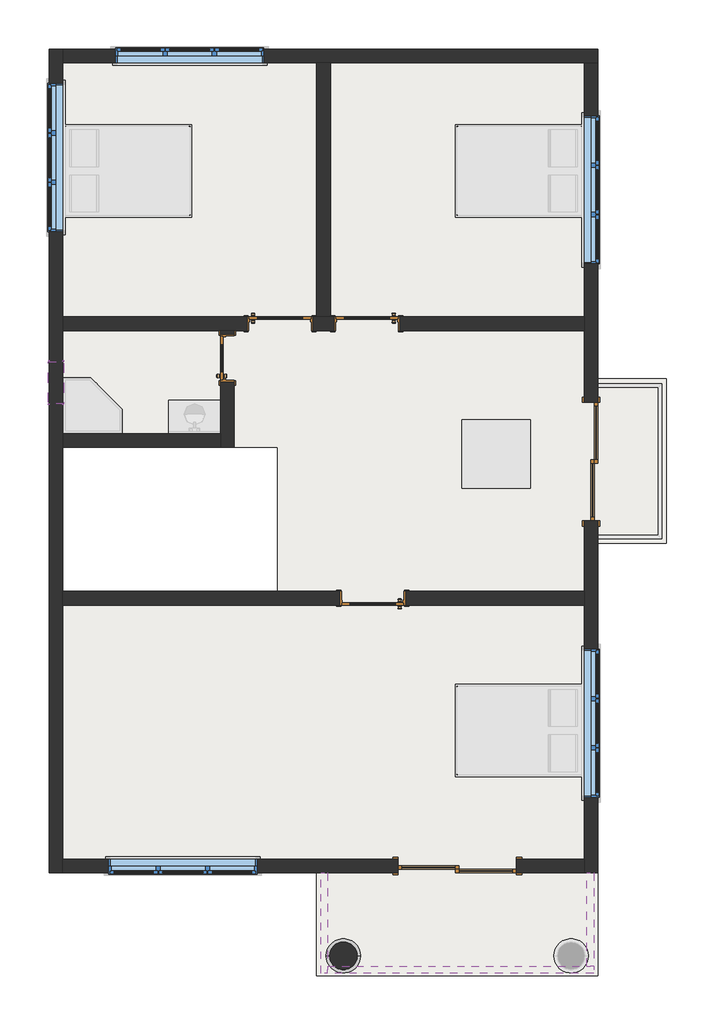
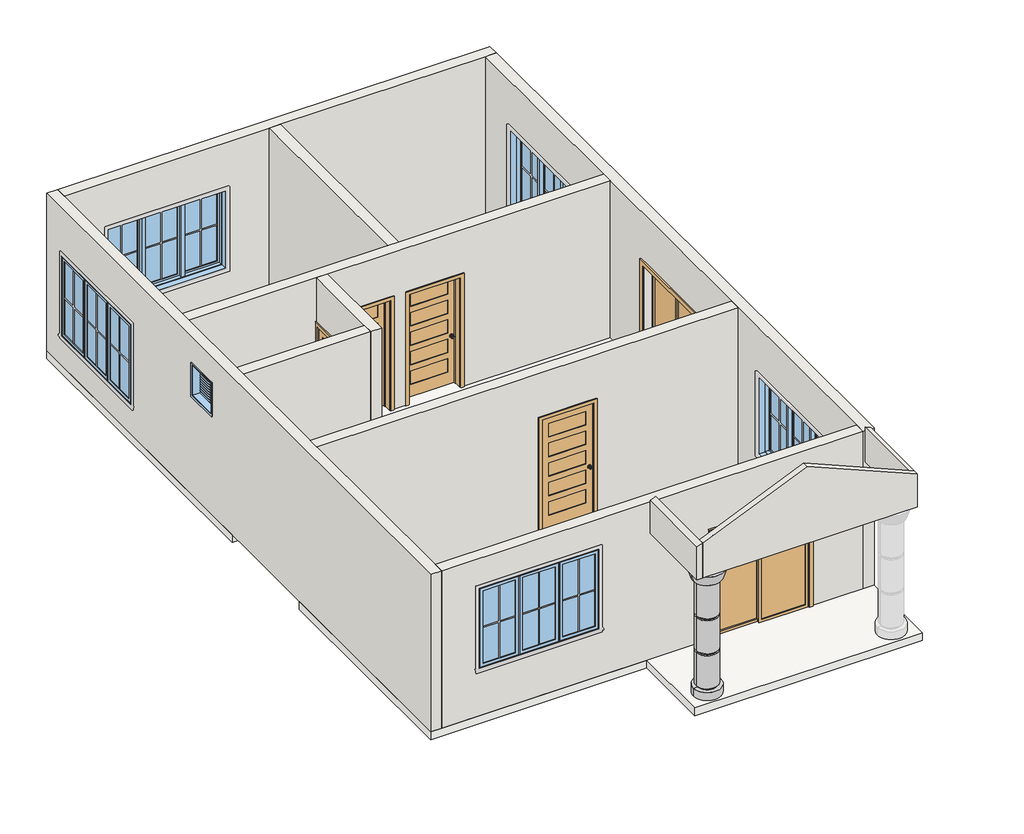
# One storey, part 1 of 2: 12 walls, 6 doors, 6 windows, 1 column, 1 slab.
"""IFC4 building model written with IfcOpenShell, lengths in millimetres."""

from ifc_helpers import new_model, si_unit, frame, origin, place, context, project, spatial, polyline, circle_curve, outline, extrude, faceted_brep, transform, mapped, element, save
from ifc_brep_helpers import plane_surface, cylinder_surface, revolved_surface, advanced_brep
from components import door_e30895c2, door_3f7a11fd, door_bc447172, door_interior_single_5_panel_vert_wood_650_x_2100_a7f2c8da, window_45599283, window_35a91c22

model = new_model("IFC4")

# Units and contexts
model_context = context("Model", 3, world=origin())
ifc_project = project(units=[si_unit("LENGTHUNIT", "METRE", prefix="MILLI")], contexts=[model_context])

# Site, building, storey
site = spatial("IfcSite", under=ifc_project)
building = spatial("IfcBuilding", under=site)
storey = spatial("IfcBuildingStorey", under=building, Elevation=3400.0)

# Column
placement = place(None, origin())
element("IfcColumn", 1, ObjectType="Metal Clad Column : 400MM COLUMN", at=placement, inside=storey, context=model_context, shape_type="AdvancedBrep", body=[
    advanced_brep(
    [(-1050.7658003, -5475.1432863, 3400.0), (-1301.5658003, -5475.1432863, 3400.0), (-799.9658003, -5475.1432863, 3400.0), (-1301.5658003, -5475.1432863, 3552.4), (-799.9658003, -5475.1432863, 3552.4), (-876.1658003, -5475.1432863, 4259.2666667), (-1225.3658003, -5475.1432863, 4259.2666667), (-1250.7658003, -5475.1432863, 4259.2666667), (-850.7658003, -5475.1432863, 4259.2666667), (-1250.7658003, -5475.1432863, 4889.9333333), (-850.7658003, -5475.1432863, 4889.9333333), (-876.1658003, -5475.1432863, 4221.1666667), (-1225.3658003, -5475.1432863, 4221.1666667), (-850.7658003, -5475.1432863, 4221.1666667), (-1250.7658003, -5475.1432863, 4221.1666667), (-850.7658003, -5475.1432863, 3590.5), (-1250.7658003, -5475.1432863, 3590.5), (-876.1658003, -5475.1432863, 3590.5), (-1225.3658003, -5475.1432863, 3590.5), (-876.1658003, -5475.1432863, 3552.4), (-1225.3658003, -5475.1432863, 3552.4), (-799.9658003, -5475.1432863, 5596.8), (-1301.5658003, -5475.1432863, 5596.8), (-1365.0658003, -5475.1432863, 5800.0), (-736.4658003, -5475.1432863, 5800.0), (-1050.7658003, -5475.1432863, 5800.0), (-876.1658003, -5475.1432863, 5596.8), (-1225.3658003, -5475.1432863, 5596.8), (-876.1658003, -5475.1432863, 5558.7), (-1225.3658003, -5475.1432863, 5558.7), (-850.7658003, -5475.1432863, 5558.7), (-1250.7658003, -5475.1432863, 5558.7), (-850.7658003, -5475.1432863, 4928.0333333), (-1250.7658003, -5475.1432863, 4928.0333333), (-876.1658003, -5475.1432863, 4928.0333333), (-1225.3658003, -5475.1432863, 4928.0333333), (-876.1658003, -5475.1432863, 4889.9333333), (-1225.3658003, -5475.1432863, 4889.9333333)],
    [
        (0, 1),
        (1, 2, circle_curve(frame((-1050.7658003, -5475.1432863, 3400.0), z_axis=(0.0, 0.0, -1.0), x_axis=(-1.0, 0.0, 0.0)), 250.8)),
        (2, 0),
        (2, 1, circle_curve(frame((-1050.7658003, -5475.1432863, 3400.0), z_axis=(0.0, 0.0, -1.0), x_axis=(-1.0, 0.0, 0.0)), 250.8)),
        (1, 3),
        (3, 4, circle_curve(frame((-1050.7658003, -5475.1432863, 3552.4), z_axis=(0.0, 0.0, -1.0), x_axis=(-1.0, 0.0, 0.0)), 250.8)),
        (4, 2),
        (4, 3, circle_curve(frame((-1050.7658003, -5475.1432863, 3552.4), z_axis=(0.0, 0.0, -1.0), x_axis=(-1.0, 0.0, 0.0)), 250.8)),
        (5, 6, circle_curve(frame((-1050.7658003, -5475.1432863, 4259.2666667), z_axis=(0.0, 0.0, 1.0), x_axis=(-1.0, 0.0, 0.0)), 174.6)),
        (6, 7),
        (7, 8, circle_curve(frame((-1050.7658003, -5475.1432863, 4259.2666667), z_axis=(0.0, 0.0, -1.0), x_axis=(-1.0, 0.0, 0.0)), 200.0)),
        (8, 5),
        (7, 9),
        (9, 10, circle_curve(frame((-1050.7658003, -5475.1432863, 4889.9333333), z_axis=(0.0, 0.0, -1.0), x_axis=(-1.0, 0.0, 0.0)), 200.0)),
        (10, 8),
        (7, 8, circle_curve(frame((-1050.7658003, -5475.1432863, 4259.2666667), z_axis=(0.0, 0.0, 1.0), x_axis=(-1.0, 0.0, 0.0)), 200.0)),
        (10, 9, circle_curve(frame((-1050.7658003, -5475.1432863, 4889.9333333), z_axis=(0.0, 0.0, -1.0), x_axis=(-1.0, 0.0, 0.0)), 200.0)),
        (6, 5, circle_curve(frame((-1050.7658003, -5475.1432863, 4259.2666667), z_axis=(0.0, 0.0, 1.0), x_axis=(-1.0, 0.0, 0.0)), 174.6)),
        (11, 12, circle_curve(frame((-1050.7658003, -5475.1432863, 4221.1666667), z_axis=(0.0, 0.0, 1.0), x_axis=(-1.0, 0.0, 0.0)), 174.6)),
        (12, 6),
        (5, 11),
        (12, 11, circle_curve(frame((-1050.7658003, -5475.1432863, 4221.1666667), z_axis=(0.0, 0.0, 1.0), x_axis=(-1.0, 0.0, 0.0)), 174.6)),
        (13, 14, circle_curve(frame((-1050.7658003, -5475.1432863, 4221.1666667), z_axis=(0.0, 0.0, 1.0), x_axis=(-1.0, 0.0, 0.0)), 200.0)),
        (14, 12),
        (11, 13),
        (14, 13, circle_curve(frame((-1050.7658003, -5475.1432863, 4221.1666667), z_axis=(0.0, 0.0, 1.0), x_axis=(-1.0, 0.0, 0.0)), 200.0)),
        (15, 16, circle_curve(frame((-1050.7658003, -5475.1432863, 3590.5), z_axis=(0.0, 0.0, 1.0), x_axis=(-1.0, 0.0, 0.0)), 200.0)),
        (16, 14),
        (13, 15),
        (16, 15, circle_curve(frame((-1050.7658003, -5475.1432863, 3590.5), z_axis=(0.0, 0.0, 1.0), x_axis=(-1.0, 0.0, 0.0)), 200.0)),
        (17, 18, circle_curve(frame((-1050.7658003, -5475.1432863, 3590.5), z_axis=(0.0, 0.0, 1.0), x_axis=(-1.0, 0.0, 0.0)), 174.6)),
        (18, 16),
        (15, 17),
        (18, 17, circle_curve(frame((-1050.7658003, -5475.1432863, 3590.5), z_axis=(0.0, 0.0, 1.0), x_axis=(-1.0, 0.0, 0.0)), 174.6)),
        (19, 20, circle_curve(frame((-1050.7658003, -5475.1432863, 3552.4), z_axis=(0.0, 0.0, 1.0), x_axis=(-1.0, 0.0, 0.0)), 174.6)),
        (20, 18),
        (17, 19),
        (20, 19, circle_curve(frame((-1050.7658003, -5475.1432863, 3552.4), z_axis=(0.0, 0.0, 1.0), x_axis=(-1.0, 0.0, 0.0)), 174.6)),
        (3, 20),
        (19, 4),
        (21, 22, circle_curve(frame((-1050.7658003, -5475.1432863, 5596.8), z_axis=(0.0, 0.0, 1.0), x_axis=(-1.0, 0.0, 0.0)), 250.8)),
        (22, 23),
        (23, 24, circle_curve(frame((-1050.7658003, -5475.1432863, 5800.0), z_axis=(0.0, 0.0, -1.0), x_axis=(-1.0, 0.0, 0.0)), 314.3)),
        (24, 21),
        (23, 25),
        (25, 24),
        (23, 24, circle_curve(frame((-1050.7658003, -5475.1432863, 5800.0), z_axis=(0.0, 0.0, 1.0), x_axis=(-1.0, 0.0, 0.0)), 314.3)),
        (22, 21, circle_curve(frame((-1050.7658003, -5475.1432863, 5596.8), z_axis=(0.0, 0.0, 1.0), x_axis=(-1.0, 0.0, 0.0)), 250.8)),
        (26, 27, circle_curve(frame((-1050.7658003, -5475.1432863, 5596.8), z_axis=(0.0, 0.0, 1.0), x_axis=(-1.0, 0.0, 0.0)), 174.6)),
        (27, 22),
        (21, 26),
        (27, 26, circle_curve(frame((-1050.7658003, -5475.1432863, 5596.8), z_axis=(0.0, 0.0, 1.0), x_axis=(-1.0, 0.0, 0.0)), 174.6)),
        (28, 29, circle_curve(frame((-1050.7658003, -5475.1432863, 5558.7), z_axis=(0.0, 0.0, 1.0), x_axis=(-1.0, 0.0, 0.0)), 174.6)),
        (29, 27),
        (26, 28),
        (29, 28, circle_curve(frame((-1050.7658003, -5475.1432863, 5558.7), z_axis=(0.0, 0.0, 1.0), x_axis=(-1.0, 0.0, 0.0)), 174.6)),
        (30, 31, circle_curve(frame((-1050.7658003, -5475.1432863, 5558.7), z_axis=(0.0, 0.0, 1.0), x_axis=(-1.0, 0.0, 0.0)), 200.0)),
        (31, 29),
        (28, 30),
        (31, 30, circle_curve(frame((-1050.7658003, -5475.1432863, 5558.7), z_axis=(0.0, 0.0, 1.0), x_axis=(-1.0, 0.0, 0.0)), 200.0)),
        (32, 33, circle_curve(frame((-1050.7658003, -5475.1432863, 4928.0333333), z_axis=(0.0, 0.0, 1.0), x_axis=(-1.0, 0.0, 0.0)), 200.0)),
        (33, 31),
        (30, 32),
        (33, 32, circle_curve(frame((-1050.7658003, -5475.1432863, 4928.0333333), z_axis=(0.0, 0.0, 1.0), x_axis=(-1.0, 0.0, 0.0)), 200.0)),
        (34, 35, circle_curve(frame((-1050.7658003, -5475.1432863, 4928.0333333), z_axis=(0.0, 0.0, 1.0), x_axis=(-1.0, 0.0, 0.0)), 174.6)),
        (35, 33),
        (32, 34),
        (35, 34, circle_curve(frame((-1050.7658003, -5475.1432863, 4928.0333333), z_axis=(0.0, 0.0, 1.0), x_axis=(-1.0, 0.0, 0.0)), 174.6)),
        (36, 37, circle_curve(frame((-1050.7658003, -5475.1432863, 4889.9333333), z_axis=(0.0, 0.0, 1.0), x_axis=(-1.0, 0.0, 0.0)), 174.6)),
        (37, 35),
        (34, 36),
        (37, 36, circle_curve(frame((-1050.7658003, -5475.1432863, 4889.9333333), z_axis=(0.0, 0.0, 1.0), x_axis=(-1.0, 0.0, 0.0)), 174.6)),
        (9, 37),
        (36, 10),
    ],
    [
        plane_surface(frame((-1050.7658003, -5475.1432863, 3400.0), z_axis=(0.0, 0.0, -1.0), x_axis=(-1.0, 0.0, 0.0))),
        cylinder_surface(frame((-1050.7658003, -5475.1432863, 5800.0), z_axis=(0.0, 0.0, -1.0), x_axis=(-1.0, 0.0, 0.0)), 250.8),
        plane_surface(frame((-1050.7658003, -5475.1432863, 4259.2666667), z_axis=(0.0, 0.0, -1.0), x_axis=(-1.0, 0.0, 0.0))),
        cylinder_surface(frame((-1050.7658003, -5475.1432863, 5800.0), z_axis=(0.0, 0.0, -1.0), x_axis=(-1.0, 0.0, 0.0)), 200.0),
        cylinder_surface(frame((-1050.7658003, -5475.1432863, 5800.0), z_axis=(0.0, 0.0, -1.0), x_axis=(-1.0, 0.0, 0.0)), 174.6),
        plane_surface(frame((-1050.7658003, -5475.1432863, 4221.1666667), z_axis=(0.0, 0.0, 1.0), x_axis=(-1.0, 0.0, 0.0))),
        plane_surface(frame((-1050.7658003, -5475.1432863, 3590.5), z_axis=(0.0, 0.0, -1.0), x_axis=(-1.0, 0.0, 0.0))),
        plane_surface(frame((-1050.7658003, -5475.1432863, 3552.4), z_axis=(0.0, 0.0, 1.0), x_axis=(-1.0, 0.0, 0.0))),
        revolved_surface(polyline([(-1365.0658003, -5475.1432863, 5800.0), (-1301.5658003, -5475.1432863, 5596.8)]), (-1050.7658003, -5475.1432863, 5800.0), (0.0, 0.0, -1.0)),
        plane_surface(frame((-1050.7658003, -5475.1432863, 5800.0), z_axis=(0.0, 0.0, 1.0), x_axis=(-1.0, 0.0, 0.0))),
        plane_surface(frame((-1050.7658003, -5475.1432863, 5596.8), z_axis=(0.0, 0.0, -1.0), x_axis=(-1.0, 0.0, 0.0))),
        plane_surface(frame((-1050.7658003, -5475.1432863, 5558.7), z_axis=(0.0, 0.0, 1.0), x_axis=(-1.0, 0.0, 0.0))),
        plane_surface(frame((-1050.7658003, -5475.1432863, 4928.0333333), z_axis=(0.0, 0.0, -1.0), x_axis=(-1.0, 0.0, 0.0))),
        plane_surface(frame((-1050.7658003, -5475.1432863, 4889.9333333), z_axis=(0.0, 0.0, 1.0), x_axis=(-1.0, 0.0, 0.0))),
    ],
    [
        (0, [[1, 2, 3]]),
        (0, [[-3, 4, -1]]),
        (1, [[-2, 5, 6, 7]]),
        (1, [[-4, -7, 8, -5]]),
        (2, [[9, 10, 11, 12]]),
        (3, [[-11, 13, 14, 15]]),
        (3, [[16, -15, 17, -13]]),
        (2, [[18, -12, -16, -10]]),
        (4, [[19, 20, -9, 21]]),
        (4, [[22, -21, -18, -20]]),
        (5, [[23, 24, -19, 25]]),
        (5, [[26, -25, -22, -24]]),
        (3, [[27, 28, -23, 29]]),
        (3, [[30, -29, -26, -28]]),
        (6, [[31, 32, -27, 33]]),
        (6, [[34, -33, -30, -32]]),
        (4, [[35, 36, -31, 37]]),
        (4, [[38, -37, -34, -36]]),
        (7, [[-6, 39, -35, 40]]),
        (7, [[-8, -40, -38, -39]]),
        (8, [[41, 42, 43, 44]]),
        (9, [[-43, 45, 46]]),
        (9, [[47, -46, -45]]),
        (8, [[48, -44, -47, -42]]),
        (10, [[49, 50, -41, 51]]),
        (10, [[52, -51, -48, -50]]),
        (4, [[53, 54, -49, 55]]),
        (4, [[56, -55, -52, -54]]),
        (11, [[57, 58, -53, 59]]),
        (11, [[60, -59, -56, -58]]),
        (3, [[61, 62, -57, 63]]),
        (3, [[64, -63, -60, -62]]),
        (12, [[65, 66, -61, 67]]),
        (12, [[68, -67, -64, -66]]),
        (4, [[69, 70, -65, 71]]),
        (4, [[72, -71, -68, -70]]),
        (13, [[-14, 73, -69, 74]]),
        (13, [[-17, -74, -72, -73]]),
    ],
),
])

# Doors
door_shape = door_e30895c2(model_context)
element("IfcDoor", 2, ObjectType="Door-Double-Sliding : 68\" x 80\"", at=placement, inside=storey, context=model_context, shape_type="MappedRepresentation", body=[
    mapped(door_shape, transform((609.2341997, -4038.1432863, 3400.0), x_axis=(-1.0, 0.0, 0.0), y_axis=(0.0, -1.0, 0.0), z_axis=(0.0, 0.0, 1.0))),
])
element("IfcDoor", 3, ObjectType="Door-Double-Sliding : 68\" x 80\"", at=placement, inside=storey, context=model_context, shape_type="MappedRepresentation", body=[
    mapped(door_shape, transform((2432.2341997, 1726.3567137, 3400.0), x_axis=(0.0, -1.0, 0.0), y_axis=(1.0, 0.0, 0.0), z_axis=(0.0, 0.0, 1.0))),
])
door_2_shape = door_3f7a11fd(model_context)
element("IfcDoor", 4, ObjectType="Door-Interior-Single-5_Panel_Vert-Wood : 36\" x 82.5\"", at=placement, inside=storey, context=model_context, shape_type="MappedRepresentation", body=[
    mapped(door_2_shape, transform((-1973.3658003, 3738.0317137, 3400.0), x_axis=(1.0, 0.0, 0.0), y_axis=(0.0, 1.0, 0.0), z_axis=(0.0, 0.0, 1.0))),
])
element("IfcDoor", 5, ObjectType="Door-Interior-Single-5_Panel_Vert-Wood : 36\" x 82.5\"", at=placement, inside=storey, context=model_context, shape_type="MappedRepresentation", body=[
    mapped(door_2_shape, transform((-623.3658003, -268.3182863, 3400.0), x_axis=(-1.0, 0.0, 0.0), y_axis=(0.0, -1.0, 0.0), z_axis=(0.0, 0.0, 1.0))),
])
door_3_shape = door_bc447172(model_context)
element("IfcDoor", 6, ObjectType="Door-Interior-Single-5_Panel_Vert-Wood : 36\" x 82.5\"", at=placement, inside=storey, context=model_context, shape_type="MappedRepresentation", body=[
    mapped(door_3_shape, transform((-708.1658003, 3738.0317137, 3400.0), x_axis=(-1.0, 0.0, 0.0), y_axis=(0.0, -1.0, 0.0), z_axis=(0.0, 0.0, 1.0))),
])
door_interior_single_5_panel_vert_wood_650_x_2100_shape = door_interior_single_5_panel_vert_wood_650_x_2100_a7f2c8da(model_context)
element("IfcDoor", 7, ObjectType="Door-Interior-Single-5_Panel_Vert-Wood : 650 x 2100", at=placement, inside=storey, context=model_context, shape_type="MappedRepresentation", body=[
    mapped(door_interior_single_5_panel_vert_wood_650_x_2100_shape, transform((-2743.9408003, 3234.4567137, 3400.0), x_axis=(0.0, 1.0, 0.0), y_axis=(-1.0, 0.0, 0.0), z_axis=(0.0, 0.0, 1.0))),
])

# Slab
element("IfcSlab", 8, ObjectType="6\" floor", at=placement, inside=storey, context=model_context, shape_type="SweptSolid", body=[
    extrude(outline(polyline([(-5340.7658003, 7734.8567137), (2659.2341997, 7734.8567137), (2659.2341997, 2934.8567137), (3659.2341997, 2934.8567137), (3659.2341997, 534.8567137), (2659.2341997, 534.8567137), (2659.2341997, -5765.1432863), (-1440.7658003, -5765.1432863), (-1440.7658003, -4265.1432863), (-5340.7658003, -4265.1432863), (-5340.7658003, -165.1432863), (-2007.1658003, -165.1432863), (-2007.1658003, 1934.8567137), (-5340.7658003, 1934.8567137), (-5340.7658003, 7734.8567137)])), frame((0.0, 0.0, 3250.0), z_axis=(0.0, 0.0, 1.0), x_axis=(1.0, 0.0, 0.0)), (0.0, 0.0, 1.0), 150.0),
])

# Walls
element("IfcWall", 9, at=placement, inside=storey, context=model_context, shape_type="Brep", body=[
    faceted_brep([(-1378.8658003, -4265.1432863, 5800.0), (-1378.8658003, -5727.0432863, 5800.0), (-1378.8658003, -5727.0432863, 6426.2749911), (-1378.8658003, -4265.1432863, 6426.2749911), (-1278.8658003, -4265.1432863, 5800.0), (-1278.8658003, -4265.1432863, 6468.7224727), (-1278.8658003, -5627.0432863, 6468.7224727), (-1278.8658003, -5727.0432863, 6468.7224727), (-1278.8658003, -5727.0432863, 5800.0), (-1278.8658003, -5627.0432863, 5800.0)], [[[0, 1, 2, 3]], [[4, 5, 6, 7, 8, 9]], [[1, 0, 4, 9, 8]], [[0, 3, 5, 4]], [[2, 1, 8, 7]], [[3, 2, 7, 6, 5]]]),
])
element("IfcWall", 10, at=placement, inside=storey, context=model_context, shape_type="Brep", body=[
    faceted_brep([(-1278.8658003, -5727.0432863, 5800.0), (2597.3341997, -5727.0432863, 5800.0), (2597.3341997, -5727.0432863, 6426.2749911), (609.2341997, -5727.0432863, 7270.1733732), (-1278.8658003, -5727.0432863, 6468.7224727), (-1278.8658003, -5627.0432863, 5800.0), (-1278.8658003, -5627.0432863, 6468.7224727), (609.2341997, -5627.0432863, 7270.1733732), (2497.3341997, -5627.0432863, 6468.7224727), (2597.3341997, -5627.0432863, 6426.2749911), (2597.3341997, -5627.0432863, 5800.0), (2497.3341997, -5627.0432863, 5800.0)], [[[0, 1, 2, 3, 4]], [[5, 6, 7, 8, 9, 10, 11]], [[1, 0, 5, 11, 10]], [[0, 4, 6, 5]], [[2, 1, 10, 9]], [[4, 3, 7, 6]], [[3, 2, 9, 8, 7]]]),
])
element("IfcWall", 11, at=placement, inside=storey, context=model_context, shape_type="SweptSolid", body=[
    extrude(outline(polyline([(5800.0, 2597.3341997), (6426.2749911, 2597.3341997), (6468.7224727, 2497.3341997), (5800.0, 2497.3341997), (5800.0, 2597.3341997)])), frame((0.0, -5627.0432863, 0.0), z_axis=(0.0, 1.0, 0.0), x_axis=(0.0, 0.0, 1.0)), (0.0, 0.0, 1.0), 1361.9),
])
element("IfcWall", 12, ObjectType="9\" wall", at=placement, inside=storey, context=model_context, shape_type="Brep", body=[
    faceted_brep([(-5140.7658003, -4265.1432863, 3400.0), (-5140.7658003, -4065.1432863, 3400.0), (-5140.7658003, -365.1432863, 3400.0), (-5140.7658003, -165.1432863, 3400.0), (-5140.7658003, 1934.8567137, 3400.0), (-5140.7658003, 2134.8567137, 3400.0), (-5140.7658003, 3634.8567137, 3400.0), (-5140.7658003, 3834.8567137, 3400.0), (-5140.7658003, 7534.8567137, 3400.0), (-5140.7658003, 7734.8567137, 3400.0), (-5140.7658003, 7734.8567137, 6400.0), (-5140.7658003, 7534.8567137, 6400.0), (-5140.7658003, 3834.8567137, 6400.0), (-5140.7658003, 3634.8567137, 6400.0), (-5140.7658003, 2134.8567137, 6400.0), (-5140.7658003, 1934.8567137, 6400.0), (-5140.7658003, -165.1432863, 6400.0), (-5140.7658003, -365.1432863, 6400.0), (-5140.7658003, -4065.1432863, 6400.0), (-5140.7658003, -4265.1432863, 6400.0), (-5140.7658003, 7234.8567137, 5512.7), (-5140.7658003, 7234.8567137, 3988.7), (-5140.7658003, 5075.8567137, 3988.7), (-5140.7658003, 5075.8567137, 5512.7), (-5140.7658003, 3180.1317137, 5909.6), (-5140.7658003, 3180.1317137, 5300.0), (-5140.7658003, 2570.5317137, 5300.0), (-5140.7658003, 2570.5317137, 5909.6), (-5340.7658003, -4265.1432863, 3400.0), (-5340.7658003, -4265.1432863, 6400.0), (-5340.7658003, 7734.8567137, 6400.0), (-5340.7658003, 7734.8567137, 3400.0), (-5340.7658003, 7234.8567137, 5512.7), (-5340.7658003, 5075.8567137, 5512.7), (-5340.7658003, 5075.8567137, 3988.7), (-5340.7658003, 7234.8567137, 3988.7), (-5340.7658003, 3180.1317137, 5909.6), (-5340.7658003, 2570.5317137, 5909.6), (-5340.7658003, 2570.5317137, 5300.0), (-5340.7658003, 3180.1317137, 5300.0)], [[[0, 1, 2, 3, 4, 5, 6, 7, 8, 9, 10, 11, 12, 13, 14, 15, 16, 17, 18, 19], [20, 21, 22, 23], [24, 25, 26, 27]], [[28, 29, 30, 31], [32, 33, 34, 35], [36, 37, 38, 39]], [[9, 8, 7, 6, 5, 4, 3, 2, 1, 0, 28, 31]], [[19, 18, 17, 16, 15, 14, 13, 12, 11, 10, 30, 29]], [[10, 9, 31, 30]], [[21, 20, 32, 35]], [[22, 21, 35, 34]], [[23, 22, 34, 33]], [[20, 23, 33, 32]], [[25, 24, 36, 39]], [[26, 25, 39, 38]], [[27, 26, 38, 37]], [[24, 27, 37, 36]], [[0, 19, 29, 28]]]),
])
element("IfcWall", 13, ObjectType="9\" wall", at=placement, inside=storey, context=model_context, shape_type="Brep", body=[
    faceted_brep([(-5140.7658003, 7534.8567137, 3400.0), (-1440.7658003, 7534.8567137, 3400.0), (-1240.7658003, 7534.8567137, 3400.0), (2459.2341997, 7534.8567137, 3400.0), (2659.2341997, 7534.8567137, 3400.0), (2659.2341997, 7534.8567137, 6400.0), (2459.2341997, 7534.8567137, 6400.0), (-1240.7658003, 7534.8567137, 6400.0), (-1440.7658003, 7534.8567137, 6400.0), (-5140.7658003, 7534.8567137, 6400.0), (-2211.2658003, 7534.8567137, 5512.7), (-2211.2658003, 7534.8567137, 3988.7), (-4370.2658003, 7534.8567137, 3988.7), (-4370.2658003, 7534.8567137, 5512.7), (-5140.7658003, 7734.8567137, 3400.0), (-5140.7658003, 7734.8567137, 6400.0), (2659.2341997, 7734.8567137, 6400.0), (2659.2341997, 7734.8567137, 3400.0), (-2211.2658003, 7734.8567137, 5512.7), (-4370.2658003, 7734.8567137, 5512.7), (-4370.2658003, 7734.8567137, 3988.7), (-2211.2658003, 7734.8567137, 3988.7)], [[[0, 1, 2, 3, 4, 5, 6, 7, 8, 9], [10, 11, 12, 13]], [[14, 15, 16, 17], [18, 19, 20, 21]], [[4, 3, 2, 1, 0, 14, 17]], [[9, 8, 7, 6, 5, 16, 15]], [[0, 9, 15, 14]], [[5, 4, 17, 16]], [[11, 10, 18, 21]], [[12, 11, 21, 20]], [[13, 12, 20, 19]], [[10, 13, 19, 18]]]),
])
element("IfcWall", 14, ObjectType="9\" wall", at=placement, inside=storey, context=model_context, shape_type="Brep", body=[
    faceted_brep([(2459.2341997, 862.7567137, 5432.0), (2459.2341997, 862.7567137, 3400.0), (2459.2341997, -165.1432863, 3400.0), (2459.2341997, -365.1432863, 3400.0), (2459.2341997, -4065.1432863, 3400.0), (2459.2341997, -4265.1432863, 3400.0), (2459.2341997, -4265.1432863, 6400.0), (2459.2341997, -4065.1432863, 6400.0), (2459.2341997, -365.1432863, 6400.0), (2459.2341997, -165.1432863, 6400.0), (2459.2341997, 3634.8567137, 6400.0), (2459.2341997, 3834.8567137, 6400.0), (2459.2341997, 7534.8567137, 6400.0), (2459.2341997, 7534.8567137, 3400.0), (2459.2341997, 3834.8567137, 3400.0), (2459.2341997, 3634.8567137, 3400.0), (2459.2341997, 2589.9567137, 3400.0), (2459.2341997, 2589.9567137, 5432.0), (2459.2341997, -3165.1432863, 5512.7), (2459.2341997, -3165.1432863, 3988.7), (2459.2341997, -1006.1432863, 3988.7), (2459.2341997, -1006.1432863, 5512.7), (2459.2341997, 4605.3567137, 5512.7), (2459.2341997, 4605.3567137, 3988.7), (2459.2341997, 6764.3567137, 3988.7), (2459.2341997, 6764.3567137, 5512.7), (2659.2341997, -4265.1432863, 3400.0), (2659.2341997, 862.7567137, 3400.0), (2659.2341997, 862.7567137, 5432.0), (2659.2341997, 2589.9567137, 5432.0), (2659.2341997, 2589.9567137, 3400.0), (2659.2341997, 7534.8567137, 3400.0), (2659.2341997, 7534.8567137, 6400.0), (2659.2341997, -4265.1432863, 6400.0), (2659.2341997, -3165.1432863, 5512.7), (2659.2341997, -1006.1432863, 5512.7), (2659.2341997, -1006.1432863, 3988.7), (2659.2341997, -3165.1432863, 3988.7), (2659.2341997, 4605.3567137, 5512.7), (2659.2341997, 6764.3567137, 5512.7), (2659.2341997, 6764.3567137, 3988.7), (2659.2341997, 4605.3567137, 3988.7)], [[[0, 1, 2, 3, 4, 5, 6, 7, 8, 9, 10, 11, 12, 13, 14, 15, 16, 17], [18, 19, 20, 21], [22, 23, 24, 25]], [[26, 27, 28, 29, 30, 31, 32, 33], [34, 35, 36, 37], [38, 39, 40, 41]], [[5, 4, 3, 2, 1, 27, 26]], [[16, 15, 14, 13, 31, 30]], [[12, 11, 10, 9, 8, 7, 6, 33, 32]], [[13, 12, 32, 31]], [[19, 18, 34, 37]], [[20, 19, 37, 36]], [[21, 20, 36, 35]], [[18, 21, 35, 34]], [[23, 22, 38, 41]], [[24, 23, 41, 40]], [[25, 24, 40, 39]], [[22, 25, 39, 38]], [[30, 29, 17, 16]], [[28, 27, 1, 0]], [[29, 28, 0, 17]], [[5, 26, 33, 6]]]),
])
element("IfcWall", 15, ObjectType="9\" wall", at=placement, inside=storey, context=model_context, shape_type="SweptSolid", body=[
    extrude(outline(polyline([(3400.0, -5140.7658003), (3400.0, -254.3658003), (5432.0, -254.3658003), (5432.0, 1472.8341997), (3400.0, 1472.8341997), (3400.0, 2459.2341997), (6400.0, 2459.2341997), (6400.0, -5140.7658003), (3400.0, -5140.7658003)]), holes=[polyline([(5838.4, -4470.2658003), (5838.4, -2311.2658003), (4314.4, -2311.2658003), (4314.4, -4470.2658003), (5838.4, -4470.2658003)])]), frame((0.0, -4265.1432863, 0.0), z_axis=(0.0, 1.0, 0.0), x_axis=(0.0, 0.0, 1.0)), (0.0, 0.0, 1.0), 200.0),
])
element("IfcWall", 16, ObjectType="9\" wall", at=placement, inside=storey, context=model_context, shape_type="Brep", body=[
    faceted_brep([(2459.2341997, 3634.8567137, 6400.0), (-2640.7658003, 3634.8567137, 6400.0), (-2840.7658003, 3634.8567137, 6400.0), (-5140.7658003, 3634.8567137, 6400.0), (-5140.7658003, 3634.8567137, 3400.0), (-2840.7658003, 3634.8567137, 3400.0), (-2640.7658003, 3634.8567137, 3400.0), (-2455.9658003, 3634.8567137, 3400.0), (-2455.9658003, 3634.8567137, 5525.4), (-1490.7658003, 3634.8567137, 5525.4), (-1490.7658003, 3634.8567137, 3400.0), (-1190.7658003, 3634.8567137, 3400.0), (-1190.7658003, 3634.8567137, 5525.4), (-225.5658003, 3634.8567137, 5525.4), (-225.5658003, 3634.8567137, 3400.0), (2459.2341997, 3634.8567137, 3400.0), (-5140.7658003, 3834.8567137, 6400.0), (-1440.7658003, 3834.8567137, 6400.0), (-1240.7658003, 3834.8567137, 6400.0), (2459.2341997, 3834.8567137, 6400.0), (2459.2341997, 3834.8567137, 3400.0), (-225.5658003, 3834.8567137, 3400.0), (-225.5658003, 3834.8567137, 5525.4), (-1190.7658003, 3834.8567137, 5525.4), (-1190.7658003, 3834.8567137, 3400.0), (-1240.7658003, 3834.8567137, 3400.0), (-1440.7658003, 3834.8567137, 3400.0), (-1490.7658003, 3834.8567137, 3400.0), (-1490.7658003, 3834.8567137, 5525.4), (-2455.9658003, 3834.8567137, 5525.4), (-2455.9658003, 3834.8567137, 3400.0), (-5140.7658003, 3834.8567137, 3400.0)], [[[0, 1, 2, 3, 4, 5, 6, 7, 8, 9, 10, 11, 12, 13, 14, 15]], [[16, 17, 18, 19, 20, 21, 22, 23, 24, 25, 26, 27, 28, 29, 30, 31]], [[4, 31, 30, 7, 6, 5]], [[20, 15, 14, 21]], [[10, 27, 26, 25, 24, 11]], [[3, 2, 1, 0, 19, 18, 17, 16]], [[4, 3, 16, 31]], [[0, 15, 20, 19]], [[9, 28, 27, 10]], [[28, 9, 8, 29]], [[29, 8, 7, 30]], [[23, 12, 11, 24]], [[12, 23, 22, 13]], [[13, 22, 21, 14]]]),
])
element("IfcWall", 17, ObjectType="9\" wall", at=placement, inside=storey, context=model_context, shape_type="SweptSolid", body=[
    extrude(outline(polyline([(6400.0, 2459.2341997), (6400.0, -5140.7658003), (3400.0, -5140.7658003), (3400.0, -1105.9658003), (5525.4, -1105.9658003), (5525.4, -140.7658003), (3400.0, -140.7658003), (3400.0, 2459.2341997), (6400.0, 2459.2341997)])), frame((0.0, -365.1432863, 0.0), z_axis=(0.0, 1.0, 0.0), x_axis=(0.0, 0.0, 1.0)), (0.0, 0.0, 1.0), 200.0),
])
element("IfcWall", 18, ObjectType="9\" wall", at=placement, inside=storey, context=model_context, shape_type="SweptSolid", body=[
    extrude(outline(polyline([(-1440.7658003, 3834.8567137), (-1440.7658003, 7534.8567137), (-1240.7658003, 7534.8567137), (-1240.7658003, 3834.8567137), (-1440.7658003, 3834.8567137)])), frame((0.0, 0.0, 3400.0), z_axis=(0.0, 0.0, 1.0), x_axis=(1.0, 0.0, 0.0)), (0.0, 0.0, 1.0), 3000.0),
])
element("IfcWall", 19, ObjectType="9\" wall", at=placement, inside=storey, context=model_context, shape_type="Brep", body=[
    faceted_brep([(-2840.7658003, 1934.8567137, 6400.0), (-2840.7658003, 2134.8567137, 6400.0), (-2840.7658003, 3634.8567137, 6400.0), (-2840.7658003, 3634.8567137, 3400.0), (-2840.7658003, 3584.8567137, 3400.0), (-2840.7658003, 3584.8567137, 5525.4), (-2840.7658003, 2884.0567137, 5525.4), (-2840.7658003, 2884.0567137, 3400.0), (-2840.7658003, 2134.8567137, 3400.0), (-2840.7658003, 1934.8567137, 3400.0), (-2640.7658003, 3634.8567137, 6400.0), (-2640.7658003, 1934.8567137, 6400.0), (-2640.7658003, 1934.8567137, 3400.0), (-2640.7658003, 2884.0567137, 3400.0), (-2640.7658003, 2884.0567137, 5525.4), (-2640.7658003, 3584.8567137, 5525.4), (-2640.7658003, 3584.8567137, 3400.0), (-2640.7658003, 3634.8567137, 3400.0)], [[[0, 1, 2, 3, 4, 5, 6, 7, 8, 9]], [[10, 11, 12, 13, 14, 15, 16, 17]], [[3, 17, 16, 4]], [[12, 9, 8, 7, 13]], [[2, 1, 0, 11, 10]], [[3, 2, 10, 17]], [[0, 9, 12, 11]], [[15, 5, 4, 16]], [[5, 15, 14, 6]], [[6, 14, 13, 7]]]),
])
element("IfcWall", 20, ObjectType="9\" wall", at=placement, inside=storey, context=model_context, shape_type="SweptSolid", body=[
    extrude(outline(polyline([(-5140.7658003, 2134.8567137), (-2840.7658003, 2134.8567137), (-2840.7658003, 1934.8567137), (-5140.7658003, 1934.8567137), (-5140.7658003, 2134.8567137)])), frame((0.0, 0.0, 3400.0), z_axis=(0.0, 0.0, 1.0), x_axis=(1.0, 0.0, 0.0)), (0.0, 0.0, 1.0), 3000.0),
])

# Windows
window_shape = window_45599283(model_context)
element("IfcWindow", 21, ObjectType="Window-Casement-Triple : 85\" x 60\"", at=placement, inside=storey, context=model_context, shape_type="MappedRepresentation", body=[
    mapped(window_shape, transform((2559.2341997, -2085.6432863, 3074.3), x_axis=(0.0, -1.0, 0.0), y_axis=(1.0, 0.0, 0.0), z_axis=(0.0, 0.0, 1.0))),
])
element("IfcWindow", 22, ObjectType="Window-Casement-Triple : 85\" x 60\"", at=placement, inside=storey, context=model_context, shape_type="MappedRepresentation", body=[
    mapped(window_shape, transform((-3290.7658003, 7634.8567137, 3074.3), x_axis=(1.0, 0.0, 0.0), y_axis=(0.0, 1.0, 0.0), z_axis=(0.0, 0.0, 1.0))),
])
element("IfcWindow", 23, ObjectType="Window-Casement-Triple : 85\" x 60\"", at=placement, inside=storey, context=model_context, shape_type="MappedRepresentation", body=[
    mapped(window_shape, transform((-5240.7658003, 6155.3567137, 3074.3), x_axis=(0.0, 1.0, 0.0), y_axis=(-1.0, 0.0, 0.0), z_axis=(0.0, 0.0, 1.0))),
])
element("IfcWindow", 24, ObjectType="Window-Casement-Triple : 85\" x 60\"", at=placement, inside=storey, context=model_context, shape_type="MappedRepresentation", body=[
    mapped(window_shape, transform((2559.2341997, 5684.8567137, 3074.3), x_axis=(0.0, -1.0, 0.0), y_axis=(1.0, 0.0, 0.0), z_axis=(0.0, 0.0, 1.0))),
])
element("IfcWindow", 25, ObjectType="Window-Casement-Triple : 85\" x 60\"", at=placement, inside=storey, context=model_context, shape_type="MappedRepresentation", body=[
    mapped(window_shape, transform((-3390.7658003, -4165.1432863, 3400.0), x_axis=(-1.0, 0.0, 0.0), y_axis=(0.0, -1.0, 0.0), z_axis=(0.0, 0.0, 1.0))),
])
window_2_shape = window_35a91c22(model_context)
element("IfcWindow", 26, ObjectType="Window-Louvers : 24\" x 24\"", at=placement, inside=storey, context=model_context, shape_type="MappedRepresentation", body=[
    mapped(window_2_shape, transform((-5234.4158003, 2875.3317137, 4385.6), x_axis=(0.0, -1.0, 0.0), y_axis=(1.0, 0.0, 0.0), z_axis=(0.0, 0.0, 1.0))),
])

save(model, "model.ifc")

# Revit data of these elements
# Type "Metal Clad Column : 400MM COLUMN"
#   Assembly Code = "B1010200"
#   Base = 0' - 6"
#   Capital = 0' - 8"
#   Diameter = 1' - 3.74803"
#   Joint Depth = 0' - 1"
#   Joint Width = 0' - 1 1/2"
#   Offset base level = 0' - 0"
#   Offset top level = 0' - 0"
#   Material = Aluminum
# Type "Door-Double-Sliding : 68\" x 80\""
#   Type Mark = "17"
#   Construction Type Id = "opn-d45"
#   Assembly Code = "C1020"
#   Analytic Construction = "Wood frame, double glass door "
#   Thickness = 0' - 2"
#   Thermal Resistance (R) = 1.8150 (h·ft²·°F)/BTU
#   Heat Transfer Coefficient (U) = 0.5510 BTU/(h·ft²·°F)
#   Height = 6' - 8"
#   Rail Width = 0' - 2"
#   Stiles = 0' - 2"
#   Trim Projection Ext = 0' - 1"
#   Trim Projection Int = 0' - 1"
#   Trim Width = 0' - 3"
#   Width = 5' - 8"
#   Define Thermal Properties by = 1
#   Glazing = Glass
#   Panel Material = Wood - Birch - Solid Stained Light Low Gloss
#   Trim Material = Paint - Sienna
#   Visual Light Transmittance = 0
#   Solar Heat Gain Coefficient = 0
#   Function = (empty or 0)
#   Wall Closure = (empty or 0)
# Type "Door-Interior-Single-5_Panel_Vert-Wood : 36\" x 82.5\""
#   Type Mark = "20"
#   Assembly Code = "C1020300"
#   Analytic Construction = "Wooden"
#   Top Rail = 0' - 4 11/16"
#   Thickness = 0' - 1 3/8"
#   Thermal Resistance (R) = 2.5876 (h·ft²·°F)/BTU
#   Swing Angle [instance default] = 90.00°
#   Stiles = 0' - 4 3/4"
#   Rough Width = 3' - 2"
#   Rough Height = 6' - 11.67717"
#   Intermediate Rail = 0' - 4 1/2"
#   Height = 6' - 10.67717"
#   Width = 3' - 0"
#   Heat Transfer Coefficient (U) = 0.3865 BTU/(h·ft²·°F)
#   Bottom Rail = 0' - 9 1/8"
#   Trim Material = Cherry
#   Panel Material = Cherry
#   Frame Material = Cherry
#   Door Handle Material = Aluminum
#   Visual Light Transmittance = 0
#   Solar Heat Gain Coefficient = 0
#   Wall Closure = (empty or 0)
#   Function = (empty or 0)
# Type "Door-Interior-Single-5_Panel_Vert-Wood : 650 x 2100"
#   Type Mark = "22"
#   Assembly Code = "C1020300"
#   Analytic Construction = "Wooden"
#   Top Rail = 0' - 4 11/16"
#   Thickness = 0' - 1 3/8"
#   Thermal Resistance (R) = 2.5876 (h·ft²·°F)/BTU
#   Swing Angle [instance default] = 90.00°
#   Stiles = 0' - 4 3/4"
#   Rough Width = 2' - 3.59055"
#   Rough Height = 6' - 11.67717"
#   Intermediate Rail = 0' - 4 1/2"
#   Height = 6' - 10.67717"
#   Width = 2' - 1.59055"
#   Heat Transfer Coefficient (U) = 0.3865 BTU/(h·ft²·°F)
#   Bottom Rail = 0' - 9 1/8"
#   Trim Material = Cherry
#   Panel Material = Cherry
#   Frame Material = Cherry
#   Door Handle Material = Aluminum
#   Visual Light Transmittance = 0
#   Solar Heat Gain Coefficient = 0
#   Wall Closure = (empty or 0)
#   Function = (empty or 0)
# Type "6\" floor"
#   Assembly Code = "B1010"
#   Function = 0
#   Layers, outside or top first: 0' - 5.90551" "MATERIAL -WHITE" (function 1)
# Type
#   Assembly Code = "B2010"
#   Layers, outside or top first: 0' - 3.93701" "MATERIAL -WHITE" (function 1)
# Type "9\" wall"
#   Assembly Code = "B2010"
#   Layers, outside or top first: 0' - 7.87402" "MATERIAL -WHITE" (function 1)
# Type "Window-Casement-Triple : 85\" x 60\""
#   Type Mark = "18"
#   Fire Rating = "0.5h"
#   Assembly Code = "B2020100"
#   Analytic Construction = "Double glazing - domestic"
#   Window Inset [instance default] = 0' - 0"
#   Wall Thickness [instance default] = 0' - 6"
#   Muntin Width = 1' - 11"
#   Visual Light Transmittance = 0.81
#   Thermal Resistance (R) = 1.8146 (h·ft²·°F)/BTU
#   Solar Heat Gain Coefficient = 0.76
#   One Third Width = 2' - 4.33333"
#   Sash Width = 2' - 3 1/2"
#   Rough Width = 7' - 1 1/2"
#   Rough Height = 5' - 0 1/2"
#   Interior Wall Closure [instance default] = 0' - 2 1/4"
#   Height = 5' - 0"
#   Heat Transfer Coefficient (U) = 0.5511 BTU/(h·ft²·°F)
#   Muntin Height = 4' - 6 1/2"
#   Frame Extension [instance default] = 0' - 0 1/4"
#   Exterior Wall Closure [instance default] = 0' - 1 1/4"
#   Extension Jamb [instance default] = 0' - 2 1/4"
#   Default Sill Height = 3' - 0"
#   Width = 7' - 1"
#   Middle Muntin Visibility = yes
#   Side Muntin Visibility = yes
#   Interior Trim Visibility [instance default] = yes
#   Exterior Trim Visibility [instance default] = yes
#   Extension Jamb Visibility [instance default] = yes
#   Muntin Pattern = Muntin Pattern_2x2 : Muntin Pattern_2x2
#   Interior Trim Material = Wood - Stained
#   Interior Trim = Trim-Window-Interior-Flat : Picture Frame
#   Interior Frame Material = Wood - Stained
#   Glass Panel Material = Glass
#   Exterior Trim Material = Clad - White
#   Exterior Trim = Trim-Window-Exterior-Flat : with Sill
#   Exterior Frame Material = Clad - White
#   Wall Closure = (empty or 0)
# Type "Window-Louvers : 24\" x 24\""
#   Type Mark = "21"
#   Construction Type Id = "GSP4R"
#   Assembly Code = "B20"
#   Analytic Construction = "1/8 in Pilkington single glazing"
#   Visual Light Transmittance = 0.9
#   Thermal Resistance (R) = 1.53941 (h·ft²·°F)/BTU
#   Solar Heat Gain Coefficient = 0.78
#   Max Height = 1' - 11.74264"
#   Height = 2' - 0"
#   Heat Transfer Coefficient (U) = 0.6496 BTU/(h·ft²·°F)
#   Blade Width [instance default] = 1' - 10 1/2"
#   Blade Vertical Thickness = 0' - 0.35355"
#   Blade Thickness = 0' - 0 1/4"
#   Blade Spacing = 0' - 1 1/2"
#   Blade Height = 0' - 1.85355"
#   Blade Depth = 0' - 3"
#   Blade Angle = 45.00°
#   Default Sill Height = 3' - 0"
#   Trim Projection_Exterior = 0' - 0 1/2"
#   Trim Projection_Interior = 0' - 0 1/2"
#   Trim Width_Exterior = 0' - 1 1/2"
#   Trim Width_Interior = 0' - 1 1/2"
#   Width = 2' - 0"
#   Max Blade Count = 12
#   Define Thermal Properties by = 1
#   Blade Count = 12
#   Frame Material = Birch
#   Louver Material = Birch
#   Trim Exterior Material = Birch
#   Trim Interior Material = Birch
#   Wall Closure = (empty or 0)
# Element 1 (IfcColumn, "Metal Clad Column : 400MM COLUMN")
#   Phase Created = New Construction
#   Materials on its faces: "Aluminum"
# Elements 2, 3 (IfcDoor, "Door-Double-Sliding : 68\" x 80\"")
#   Phase Created = New Construction
#   Materials on its faces: "Paint - Sienna", "Wood - Birch - Solid Stained Light Low Gloss", "Glass"
# Element 4 (IfcDoor, "Door-Interior-Single-5_Panel_Vert-Wood : 36\" x 82.5\"")
#   Phase Created = New Construction
#   Materials on its faces: "Cherry", "Aluminum"
# Elements 5, 6 (IfcDoor, "Door-Interior-Single-5_Panel_Vert-Wood : 36\" x 82.5\"")
#   Swing Angle = 90.00°
#   Phase Created = New Construction
#   Materials on its faces: "Cherry", "Aluminum"
# Element 7 (IfcDoor, "Door-Interior-Single-5_Panel_Vert-Wood : 650 x 2100")
#   Swing Angle = 90.00°
#   Phase Created = New Construction
#   Materials on its faces: "Cherry", "Aluminum"
# Element 8 (IfcSlab, "6\" floor")
#   built-in parameter 1001955 = 3.14159 (stored number, unit not read)
#   Height Offset From Level = 0' - 0"
#   Phase Created = New Construction
#   Materials on its faces: "MATERIAL -WHITE"
# Elements 9, 10, 11 (IfcWall)
#   built-in parameter 1001111 = 7' - 10.48819"
#   Top Offset = 0' - 0"
#   Base Offset = 7' - 10.48819"
#   wall height = 1' - 11.62205"
#   Phase Created = New Construction
#   Top Constraint = 3rd Roof .L
#   Materials on its faces: "MATERIAL -WHITE"
# Elements 12, 13, 14, 15, 16, 17, 18, 19, 20 (IfcWall, "9\" wall")
#   Top Offset = 0' - 0"
#   Base Offset = 0' - 0"
#   wall height = 9' - 10.11024"
#   Phase Created = New Construction
#   Top Constraint = 3rd Roof .L
#   Materials on its faces: "MATERIAL -WHITE"
# Element 21 (IfcWindow, "Window-Casement-Triple : 85\" x 60\"")
#   Mark = "7"
#   Window Inset = 0' - 0"
#   Interior Wall Closure = 0' - 2 1/4"
#   Frame Extension = 0' - 0 1/4"
#   Exterior Wall Closure = 0' - 1 1/4"
#   Interior Trim Visibility = yes
#   Exterior Trim Visibility = yes
#   Phase Created = New Construction
#   Materials on its faces: "Wood - Stained", "Glass", "Clad - White"
# Element 22 (IfcWindow, "Window-Casement-Triple : 85\" x 60\"")
#   Mark = "8"
#   Window Inset = 0' - 0"
#   Interior Wall Closure = 0' - 2 1/4"
#   Frame Extension = 0' - 0 1/4"
#   Exterior Wall Closure = 0' - 1 1/4"
#   Interior Trim Visibility = yes
#   Exterior Trim Visibility = yes
#   Phase Created = New Construction
#   Materials on its faces: "Wood - Stained", "Glass", "Clad - White"
# Element 23 (IfcWindow, "Window-Casement-Triple : 85\" x 60\"")
#   Mark = "9"
#   Window Inset = 0' - 0"
#   Interior Wall Closure = 0' - 2 1/4"
#   Frame Extension = 0' - 0 1/4"
#   Exterior Wall Closure = 0' - 1 1/4"
#   Interior Trim Visibility = yes
#   Exterior Trim Visibility = yes
#   Phase Created = New Construction
#   Materials on its faces: "Wood - Stained", "Glass", "Clad - White"
# Element 24 (IfcWindow, "Window-Casement-Triple : 85\" x 60\"")
#   Mark = "12"
#   Window Inset = 0' - 0"
#   Interior Wall Closure = 0' - 2 1/4"
#   Frame Extension = 0' - 0 1/4"
#   Exterior Wall Closure = 0' - 1 1/4"
#   Interior Trim Visibility = yes
#   Exterior Trim Visibility = yes
#   Phase Created = New Construction
#   Materials on its faces: "Wood - Stained", "Glass", "Clad - White"
# Element 25 (IfcWindow, "Window-Casement-Triple : 85\" x 60\"")
#   Mark = "13"
#   Window Inset = 0' - 0"
#   Interior Wall Closure = 0' - 2 1/4"
#   Frame Extension = 0' - 0 1/4"
#   Exterior Wall Closure = 0' - 1 1/4"
#   Interior Trim Visibility = yes
#   Exterior Trim Visibility = yes
#   Phase Created = New Construction
#   Materials on its faces: "Wood - Stained", "Glass", "Clad - White"
# Element 26 (IfcWindow, "Window-Louvers : 24\" x 24\"")
#   Mark = "11"
#   Blade Width = 1' - 10 1/2"
#   Phase Created = New Construction
#   Materials on its faces: "Birch"
# Materials
#   "Aluminum": class "Metal", colour RGB 247 247 247, transparency 0, Description = "Aluminum 6061", Cost = 0
#   "Glass": class "Glass", colour RGB 0 128 192, transparency 0.75, Description = "Soda Lime Glass", Cost = 0
#   "Wood - Birch - Solid Stained Light Low Gloss": class "Wood", colour RGB 210 159 95, transparency 0, Cost = 0
#   "Paint - Sienna": colour RGB 118 70 51, transparency 0, Cost = 0
#   "Cherry": class "Wood", colour RGB 226 177 128, transparency 0, Description = "Prunus Serotina", Cost = 0
#   "MATERIAL -WHITE": class "Generic", colour RGB 255 255 255, transparency 0, Cost = 0
#   "Wood - Stained": class "Wood", colour RGB 224 178 126, transparency 0, Cost = 0
#   "Clad - White": class "Wood", colour RGB 242 242 238, transparency 0, Cost = 0
#   "Birch": class "Wood", colour RGB 224 178 126, transparency 0, Description = "Betula Alleghaniensis", Cost = 0
